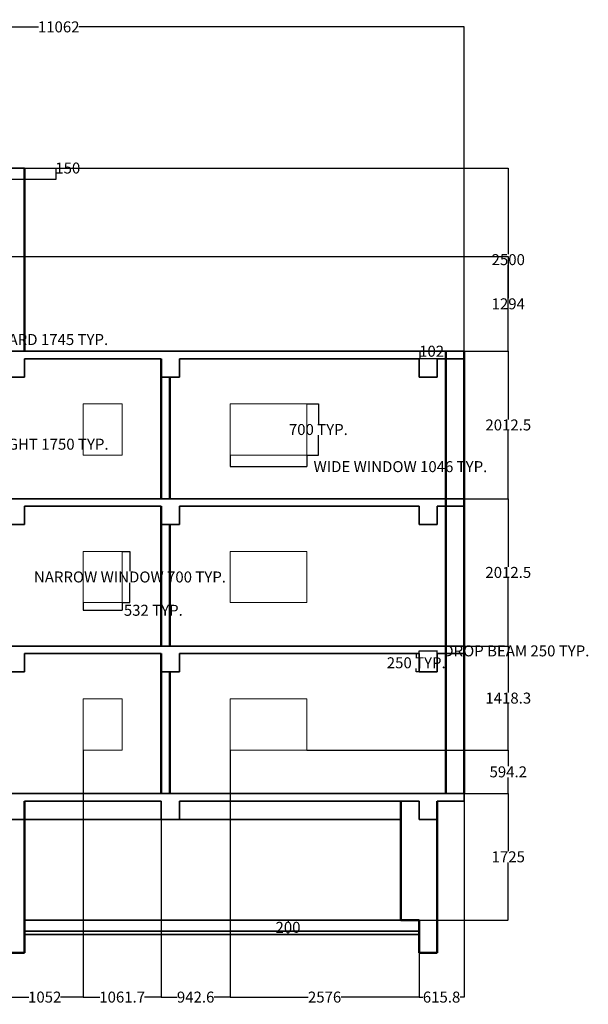
# Model space of a CAD drawing. Units: millimetres. Extents: x -1193 to 12449, y -949 to 12489.
# Tile 2 of 2: x 4692 to 12449, y -949 to 12489. Entities that reach past the tile are written whole.
import ezdxf

# ---------------------------------------------------------------- set-up
doc = ezdxf.new("R2010")
doc.units = ezdxf.units.MM
doc.header["$LTSCALE"] = 12
doc.header["$MEASUREMENT"] = 0
for name, color, linetype, lineweight in [('A-ANNO-DIMS', 2, 'Continuous', 18), ('A-FLOR', 7, 'Continuous', 35), ('A-GLAZ', 4, 'Continuous', 18), ('A-ROOF', 7, 'Continuous', 35), ('A-WALL', 7, 'Continuous', 50), ('S-BEAM', 1, 'Continuous', 35), ('S-COLS', 1, 'Continuous', 50), ('S-FNDN', 1, 'Continuous', 50)]:
    doc.layers.add(name, color=color, linetype=linetype, lineweight=lineweight)
doc.styles.get("Standard").update_dxf_attribs({"font": 'arial.ttf'})
doc.dimstyles.get("Standard").update_dxf_attribs({"dimtxt": 150, "dimasz": 0.18, "dimexe": 0.18, "dimexo": 0.0625, "dimgap": 0.09, "dimtad": 0, "dimtih": 1, "dimtoh": 1, "dimdec": 0, "dimzin": 0, "dimdsep": 46, "dimtxsty": 'Standard', "dimcen": 0.09, "dimadec": 0, "dimazin": 0, "dimtfac": 1, "dimtdec": 0, "dimtofl": 0, "dimtmove": 0, "dimatfit": 3, "dimfxl": 1, "dimtolj": 1, "dimtzin": 0, "dimarcsym": 0})

# ---------------------------------------------------------------- blocks, each defined once
blk = doc.blocks.new('*D4')
at = {"layer": 'A-ANNO-DIMS', "color": 0, "lineweight": -2, "ltscale": 8, "transparency": 16777216}
for p, q in [((8280.605673072427, 201.7493925244232), (8352.514123086432, 201.7493925244232)), ((8352.334123086432, 201.5693925244232), (8352.334123086432, 178.4253406826769)), ((8280.605673072427, 1.749392524423062), (8352.514123086432, 1.749392524423074)), ((8352.334123086432, 1.929392524423073), (8352.334123086432, 25.07344436616934))]:
    blk.add_line(p, q, dxfattribs=at)
at = {"layer": 'A-ANNO-DIMS', "color": 0, "ltscale": 8, "transparency": 16777216}
for points in [[(8352.304123086431, 201.5693925244232), (8352.364123086432, 201.5693925244232), (8352.334123086432, 201.7493925244232)], [(8352.304123086431, 1.929392524423073), (8352.364123086432, 1.929392524423073), (8352.334123086432, 1.749392524423073)]]:
    blk.add_solid(points, dxfattribs=at)
at = {"layer": 'Defpoints', "color": 0, "ltscale": 8, "transparency": 16777216}
for p in [(8280.543173072427, 201.7493925244232), (8280.543173072427, 1.749392524423062), (8352.334123086432, 1.749392524423073)]:
    blk.add_point(p, dxfattribs=at)
at = {"layer": 'A-ANNO-DIMS', "color": 0, "ltscale": 8, "transparency": 16777216, "insert": (8352.33412308643, 101.7493925244207), "char_height": 150, "attachment_point": 5}
blk.add_mtext('\\A1;200', dxfattribs=at)
blk = doc.blocks.new('*D7')
at = {"layer": 'A-ANNO-DIMS', "color": 0, "lineweight": -2, "ltscale": 8, "transparency": 16777216}
for p, q in [((4507.073797115451, 10464.24939252442), (5189.656778496646, 10464.24939252442)), ((5189.476778496646, 10464.24939252442), (5189.476778496646, 10464.42939252443)), ((5189.476778496646, 10464.42939252443), (5189.656778496646, 10464.42939252443)), ((5189.476778496646, 10314.42939252443), (5189.476778496646, 10464.06939252442)), ((4507.073797115451, 10314.24939252443), (5189.656778496646, 10314.24939252443))]:
    blk.add_line(p, q, dxfattribs=at)
at = {"layer": 'A-ANNO-DIMS', "color": 0, "ltscale": 8, "transparency": 16777216}
for points in [[(5189.446778496646, 10464.06939252442), (5189.506778496646, 10464.06939252442), (5189.476778496646, 10464.24939252442)], [(5189.446778496646, 10314.42939252443), (5189.506778496646, 10314.42939252443), (5189.476778496646, 10314.24939252443)]]:
    blk.add_solid(points, dxfattribs=at)
at = {"layer": 'Defpoints', "color": 0, "ltscale": 8, "transparency": 16777216}
for p in [(4507.01129711545, 10464.24939252442), (5189.476778496646, 10464.24939252442), (4507.01129711545, 10314.24939252443)]:
    blk.add_point(p, dxfattribs=at)
at = {"layer": 'A-ANNO-DIMS', "color": 0, "ltscale": 8, "transparency": 16777216, "insert": (5348.136955849991, 10464.42939252442), "char_height": 150, "attachment_point": 5}
blk.add_mtext('\\A1;150', dxfattribs=at)
blk = doc.blocks.new('WIN-NARROW-ELEV')
at = {"ltscale": 8}
blk.add_lwpolyline([(0, 699.7375599981679), (532.1917753348897, 699.7375599981679), (532.1917753348897, 0), (0, 0)], close=True, dxfattribs=at)
blk = doc.blocks.new('WIN-WIDE-ELEV')
at = {"ltscale": 8}
blk.add_lwpolyline([(0, 699.7375599981679), (1046.240615612791, 699.7375599981679), (1046.240615612791, 0), (0, 0)], close=True, dxfattribs=at)
blk = doc.blocks.new('BEAM-DROP-250x250')
for p, q in [((0, 250), (0, 0)), ((250, 0), (250, 250)), ((0, 0), (250, 0))]:
    blk.add_line(p, q)
blk = doc.blocks.new('*D15')
at = {"layer": 'A-ANNO-DIMS', "color": 0, "lineweight": -2, "ltscale": 8, "transparency": 16777216}
for p, q in [((10139.29307540164, 3837.311892524423), (10139.29307540164, 3874.929392524423)), ((10139.47307540164, 3874.749392524423), (10389.11307540164, 3874.749392524423)), ((10389.29307540164, 3837.311892524423), (10389.29307540164, 3874.929392524423)), ((10389.29307540164, 3874.749392524423), (10389.47307540164, 3874.749392524423))]:
    blk.add_line(p, q, dxfattribs=at)
at = {"layer": 'A-ANNO-DIMS', "color": 0, "ltscale": 8, "transparency": 16777216}
for points in [[(10139.47307540164, 3874.779392524423), (10139.47307540164, 3874.719392524422), (10139.29307540164, 3874.749392524423)], [(10389.11307540164, 3874.779392524423), (10389.11307540164, 3874.719392524422), (10389.29307540164, 3874.749392524423)]]:
    blk.add_solid(points, dxfattribs=at)
at = {"layer": 'Defpoints', "color": 0, "ltscale": 8, "transparency": 16777216}
for p in [(10139.29307540164, 3837.249392524423), (10389.29307540164, 3874.749392524423), (10389.29307540164, 3837.249392524423)]:
    blk.add_point(p, dxfattribs=at)
at = {"layer": 'A-ANNO-DIMS', "color": 0, "ltscale": 8, "transparency": 16777216, "insert": (11467.03579027203, 3874.749392524423), "char_height": 150, "attachment_point": 5}
blk.add_mtext('\\A1;DROP BEAM 250 TYP.', dxfattribs=at)
blk = doc.blocks.new('*D16')
at = {"layer": 'A-ANNO-DIMS', "color": 0, "lineweight": -2, "ltscale": 8, "transparency": 16777216}
for p, q in [((10139.23057540164, 3837.249392524425), (10101.61307540164, 3837.249392524425)), ((10101.79307540165, 3837.069392524425), (10101.79307540165, 3788.925340682679)), ((10101.79307540165, 3587.429392524425), (10101.79307540165, 3635.573444366171)), ((10139.23057540164, 3587.249392524425), (10101.61307540164, 3587.249392524425))]:
    blk.add_line(p, q, dxfattribs=at)
at = {"layer": 'A-ANNO-DIMS', "color": 0, "ltscale": 8, "transparency": 16777216}
for points in [[(10101.76307540164, 3837.069392524425), (10101.82307540165, 3837.069392524425), (10101.79307540165, 3837.249392524425)], [(10101.76307540164, 3587.429392524425), (10101.82307540165, 3587.429392524425), (10101.79307540165, 3587.249392524425)]]:
    blk.add_solid(points, dxfattribs=at)
at = {"layer": 'Defpoints', "color": 0, "ltscale": 8, "transparency": 16777216}
for p in [(10101.79307540165, 3837.249392524425), (10139.29307540164, 3837.249392524425), (10139.29307540164, 3587.249392524425)]:
    blk.add_point(p, dxfattribs=at)
at = {"layer": 'A-ANNO-DIMS', "color": 0, "ltscale": 8, "transparency": 16777216, "insert": (10101.79307540164, 3712.249392524422), "char_height": 150, "attachment_point": 5}
blk.add_mtext('\\A1;250 TYP.', dxfattribs=at)
blk = doc.blocks.new('*D19')
at = {"layer": 'A-ANNO-DIMS', "color": 0, "lineweight": -2, "ltscale": 8, "transparency": 16777216}
for p, q in [((1557.011297115448, 6957.936892524424), (1557.011297115448, 6695.319392524424)), ((3307.01129711545, 6957.936892524424), (3307.01129711545, 6695.319392524424)), ((1557.191297115448, 6695.499392524424), (3306.831297115449, 6695.499392524424)), ((3307.01129711545, 6695.499392524424), (3307.19129711545, 6695.499392524424))]:
    blk.add_line(p, q, dxfattribs=at)
at = {"layer": 'A-ANNO-DIMS', "color": 0, "ltscale": 8, "transparency": 16777216}
for points in [[(1557.191297115448, 6695.529392524425), (1557.191297115448, 6695.469392524424), (1557.011297115448, 6695.499392524424)], [(3306.831297115449, 6695.529392524425), (3306.831297115449, 6695.469392524424), (3307.01129711545, 6695.499392524424)]]:
    blk.add_solid(points, dxfattribs=at)
at = {"layer": 'Defpoints', "color": 0, "ltscale": 8, "transparency": 16777216}
for p in [(1557.011297115448, 6957.999392524424), (3307.01129711545, 6957.999392524424), (3307.01129711545, 6695.499392524424)]:
    blk.add_point(p, dxfattribs=at)
at = {"layer": 'A-ANNO-DIMS', "color": 0, "ltscale": 8, "transparency": 16777216, "insert": (4652.318814168655, 6695.499392524424), "char_height": 150, "attachment_point": 5}
blk.add_mtext('\\A1;RETURN FLIGHT 1750 TYP.', dxfattribs=at)
blk = doc.blocks.new('*D21')
at = {"layer": 'A-ANNO-DIMS', "color": 0, "lineweight": -2, "ltscale": 8, "transparency": 16777216}
for p, q in [((1557.011297115448, 7862.311892524418), (1557.011297115448, 8124.17479182941)), ((1557.191297115448, 8123.99479182941), (3301.800625815397, 8123.99479182941)), ((3301.980625815397, 7862.311892524418), (3301.980625815397, 8124.17479182941)), ((3301.980625815397, 8123.99479182941), (3302.160625815397, 8123.99479182941))]:
    blk.add_line(p, q, dxfattribs=at)
at = {"layer": 'A-ANNO-DIMS', "color": 0, "ltscale": 8, "transparency": 16777216}
for points in [[(1557.191297115448, 8124.024791829411), (1557.191297115448, 8123.964791829411), (1557.011297115448, 8123.99479182941)], [(3301.800625815397, 8124.024791829411), (3301.800625815397, 8123.964791829411), (3301.980625815397, 8123.99479182941)]]:
    blk.add_solid(points, dxfattribs=at)
at = {"layer": 'Defpoints', "color": 0, "ltscale": 8, "transparency": 16777216}
for p in [(3301.980625815397, 8123.99479182941), (1557.011297115448, 7862.249392524418), (3301.980625815397, 7862.249392524418)]:
    blk.add_point(p, dxfattribs=at)
at = {"layer": 'A-ANNO-DIMS', "color": 0, "ltscale": 8, "transparency": 16777216, "insert": (4653.120339321535, 8123.99479182941), "char_height": 150, "attachment_point": 5}
blk.add_mtext('\\A1;RETURN GUARD 1745 TYP.', dxfattribs=at)
blk = doc.blocks.new('*D23')
at = {"layer": 'A-ANNO-DIMS', "color": 0, "lineweight": -2, "ltscale": 8, "transparency": 16777216}
for p, q in [((6091.350578652216, 5233.211343509282), (6196.428712651947, 5233.211343509282)), ((6196.248712651946, 5233.031343509281), (6196.248712651946, 4961.041704028616)), ((6196.248712651946, 4533.653783511115), (6196.248712651946, 4805.643422991781)), ((6091.350578652216, 4533.473783511113), (6196.428712651947, 4533.473783511115))]:
    blk.add_line(p, q, dxfattribs=at)
at = {"layer": 'A-ANNO-DIMS', "color": 0, "ltscale": 8, "transparency": 16777216}
for points in [[(6196.218712651947, 5233.031343509281), (6196.278712651946, 5233.031343509281), (6196.248712651946, 5233.211343509282)], [(6196.218712651947, 4533.653783511115), (6196.278712651946, 4533.653783511115), (6196.248712651946, 4533.473783511115)]]:
    blk.add_solid(points, dxfattribs=at)
at = {"layer": 'Defpoints', "color": 0, "ltscale": 8, "transparency": 16777216}
for p in [(6091.288078652215, 5233.211343509282), (6196.248712651946, 5233.211343509282), (6091.288078652215, 4533.473783511113)]:
    blk.add_point(p, dxfattribs=at)
at = {"layer": 'A-ANNO-DIMS', "color": 0, "ltscale": 8, "transparency": 16777216, "insert": (6196.248712651946, 4883.342563510196), "char_height": 150, "attachment_point": 5}
blk.add_mtext('\\A1;NARROW WINDOW 700 TYP.', dxfattribs=at)
blk = doc.blocks.new('*D24')
at = {"layer": 'A-ANNO-DIMS', "color": 0, "lineweight": -2, "ltscale": 8, "transparency": 16777216}
for p, q in [((5559.096303317324, 4533.411283511112), (5559.096303317324, 4428.333149511386)), ((6091.288078652214, 4533.411283511112), (6091.288078652214, 4428.333149511386)), ((5559.276303317324, 4428.513149511386), (6091.108078652213, 4428.513149511386)), ((6091.288078652214, 4428.513149511386), (6091.468078652214, 4428.513149511386))]:
    blk.add_line(p, q, dxfattribs=at)
at = {"layer": 'A-ANNO-DIMS', "color": 0, "ltscale": 8, "transparency": 16777216}
for points in [[(5559.276303317324, 4428.543149511386), (5559.276303317324, 4428.483149511387), (5559.096303317324, 4428.513149511386)], [(6091.108078652213, 4428.543149511386), (6091.108078652213, 4428.483149511387), (6091.288078652214, 4428.513149511386)]]:
    blk.add_solid(points, dxfattribs=at)
at = {"layer": 'Defpoints', "color": 0, "ltscale": 8, "transparency": 16777216}
for p in [(5559.096303317324, 4533.473783511111), (6091.288078652214, 4533.473783511111), (6091.288078652214, 4428.513149511386)]:
    blk.add_point(p, dxfattribs=at)
at = {"layer": 'A-ANNO-DIMS', "color": 0, "ltscale": 8, "transparency": 16777216, "insert": (6514.903917669949, 4428.513149511386), "char_height": 150, "attachment_point": 5}
blk.add_mtext('\\A1;532 TYP.', dxfattribs=at)
blk = doc.blocks.new('*D25')
at = {"layer": 'A-ANNO-DIMS', "color": 0, "lineweight": -2, "ltscale": 8, "transparency": 16777216}
for p, q in [((7563.33082917866, 6545.911283511111), (7563.33082917866, 6388.857691169192)), ((8609.57144479145, 6545.911283511111), (8609.57144479145, 6388.857691169192)), ((7563.51082917866, 6389.037691169193), (8609.39144479145, 6389.037691169193)), ((8609.57144479145, 6389.037691169193), (8609.75144479145, 6389.037691169193))]:
    blk.add_line(p, q, dxfattribs=at)
at = {"layer": 'A-ANNO-DIMS', "color": 0, "ltscale": 8, "transparency": 16777216}
for points in [[(7563.51082917866, 6389.067691169192), (7563.51082917866, 6389.007691169194), (7563.33082917866, 6389.037691169193)], [(8609.39144479145, 6389.067691169192), (8609.39144479145, 6389.007691169194), (8609.57144479145, 6389.037691169193)]]:
    blk.add_solid(points, dxfattribs=at)
at = {"layer": 'Defpoints', "color": 0, "ltscale": 8, "transparency": 16777216}
for p in [(7563.33082917866, 6545.973783511112), (8609.57144479145, 6545.973783511112), (8609.57144479145, 6389.037691169193)]:
    blk.add_point(p, dxfattribs=at)
at = {"layer": 'A-ANNO-DIMS', "color": 0, "ltscale": 8, "transparency": 16777216, "insert": (9886.018116005638, 6389.037691169193), "char_height": 150, "attachment_point": 5}
blk.add_mtext('\\A1;WIDE WINDOW 1046 TYP.', dxfattribs=at)
blk = doc.blocks.new('*D26')
at = {"layer": 'A-ANNO-DIMS', "color": 0, "lineweight": -2, "ltscale": 8, "transparency": 16777216}
for p, q in [((8609.633944791454, 7245.711343509284), (8766.687537133377, 7245.711343509284)), ((8766.507537133377, 7245.531343509283), (8766.507537133377, 6972.518511668453)), ((8766.507537133377, 6546.153783511115), (8766.507537133377, 6819.166615351945)), ((8609.633944791454, 6545.973783511115), (8766.687537133377, 6545.973783511115))]:
    blk.add_line(p, q, dxfattribs=at)
at = {"layer": 'A-ANNO-DIMS', "color": 0, "ltscale": 8, "transparency": 16777216}
for points in [[(8766.477537133376, 7245.531343509283), (8766.53753713338, 7245.531343509283), (8766.507537133377, 7245.711343509284)], [(8766.477537133376, 6546.153783511115), (8766.53753713338, 6546.153783511115), (8766.507537133377, 6545.973783511115)]]:
    blk.add_solid(points, dxfattribs=at)
at = {"layer": 'Defpoints', "color": 0, "ltscale": 8, "transparency": 16777216}
for p in [(8609.571444791454, 7245.711343509284), (8766.507537133377, 7245.711343509284), (8609.571444791454, 6545.973783511115)]:
    blk.add_point(p, dxfattribs=at)
at = {"layer": 'A-ANNO-DIMS', "color": 0, "ltscale": 8, "transparency": 16777216, "insert": (8766.507537133377, 6895.842563510194), "char_height": 150, "attachment_point": 5}
blk.add_mtext('\\A1;700 TYP.', dxfattribs=at)
blk = doc.blocks.new('*D27')
at = {"layer": 'A-ANNO-DIMS', "color": 0, "lineweight": -2, "ltscale": 8, "transparency": 16777216}
for p, q in [((-307.014113, 8654.059893999998), (-307.0141129999998, 12390.66548)), ((-306.8341129999998, 12390.48548), (4949.545781004093, 12390.48548)), ((10754.946057, 12390.48548), (5498.566162995907, 12390.48548)), ((10755.126057, 7964.311893), (10755.126057, 12390.66548))]:
    blk.add_line(p, q, dxfattribs=at)
at = {"layer": 'A-ANNO-DIMS', "color": 0, "ltscale": 8, "transparency": 16777216}
for points in [[(-306.8341129999998, 12390.51548), (-306.8341129999998, 12390.45548), (-307.0141129999998, 12390.48548)], [(10754.946057, 12390.51548), (10754.946057, 12390.45548), (10755.126057, 12390.48548)]]:
    blk.add_solid(points, dxfattribs=at)
at = {"layer": 'Defpoints', "color": 0, "ltscale": 8, "transparency": 16777216}
for p in [(10755.126057, 12390.48548), (-307.014113, 8653.997393999998), (10755.126057, 7964.249393)]:
    blk.add_point(p, dxfattribs=at)
at = {"layer": 'A-ANNO-DIMS', "color": 0, "ltscale": 8, "transparency": 16777216, "insert": (5224.055972, 12390.48548), "char_height": 150, "attachment_point": 5}
blk.add_mtext('\\A1;11062', dxfattribs=at)
blk = doc.blocks.new('*D30')
at = {"layer": 'A-ANNO-DIMS', "color": 0, "lineweight": -2, "ltscale": 8, "transparency": 16777216}
for p, q in [((5559.096303, 2520.911284), (5559.096303, -850.4306069999998)), ((4507.011297, -248.313107), (4507.011297, -850.430607)), ((4507.191297000001, -850.250607), (4816.814413915416, -850.250607)), ((5558.916303, -850.250607), (5249.293186084583, -850.250607))]:
    blk.add_line(p, q, dxfattribs=at)
at = {"layer": 'A-ANNO-DIMS', "color": 0, "ltscale": 8, "transparency": 16777216}
for points in [[(4507.191297000001, -850.2206069999999), (4507.191297000001, -850.280607), (4507.011297, -850.250607)], [(5558.916303, -850.2206069999999), (5558.916303, -850.280607), (5559.096303, -850.250607)]]:
    blk.add_solid(points, dxfattribs=at)
at = {"layer": 'Defpoints', "color": 0, "ltscale": 8, "transparency": 16777216}
for p in [(5559.096303, 2520.973784), (4507.011297, -248.250607), (5559.096303, -850.250607)]:
    blk.add_point(p, dxfattribs=at)
at = {"layer": 'A-ANNO-DIMS', "color": 0, "ltscale": 8, "transparency": 16777216, "insert": (5033.0538, -850.250607), "char_height": 150, "attachment_point": 5}
blk.add_mtext('\\A1;1052', dxfattribs=at)
blk = doc.blocks.new('*D31')
at = {"layer": 'A-ANNO-DIMS', "color": 0, "lineweight": -2, "ltscale": 8, "transparency": 16777216}
for p, q in [((5559.096303, 2520.911284), (5559.096303, -850.4306069999998)), ((6620.771954, 1575.086893), (6620.771954, -850.4306069999994)), ((5559.276303, -850.250607), (5785.546720587313, -850.250607)), ((6620.591954, -850.250607), (6394.321536412687, -850.250607))]:
    blk.add_line(p, q, dxfattribs=at)
at = {"layer": 'A-ANNO-DIMS', "color": 0, "ltscale": 8, "transparency": 16777216}
for points in [[(5559.276303, -850.2206069999999), (5559.276303, -850.280607), (5559.096303, -850.250607)], [(6620.591954, -850.2206069999999), (6620.591954, -850.280607), (6620.771954, -850.250607)]]:
    blk.add_solid(points, dxfattribs=at)
at = {"layer": 'Defpoints', "color": 0, "ltscale": 8, "transparency": 16777216}
for p in [(5559.096303, 2520.973784), (6620.771954, 1575.149393), (6620.771954, -850.250607)]:
    blk.add_point(p, dxfattribs=at)
at = {"layer": 'A-ANNO-DIMS', "color": 0, "ltscale": 8, "transparency": 16777216, "insert": (6089.9341285, -850.250607), "char_height": 150, "attachment_point": 5}
blk.add_mtext('\\A1;1061.7', dxfattribs=at)
blk = doc.blocks.new('*D32')
at = {"layer": 'A-ANNO-DIMS', "color": 0, "lineweight": -2, "ltscale": 8, "transparency": 16777216}
for p, q in [((7563.330829, 2520.911284), (7563.330829, -850.4306069999998)), ((6620.771954, 1575.086893), (6620.771954, -850.4306069999994)), ((6620.951954, -850.250607), (6838.925920831513, -850.250607)), ((7563.150829, -850.250607), (7345.176862168486, -850.250607))]:
    blk.add_line(p, q, dxfattribs=at)
at = {"layer": 'A-ANNO-DIMS', "color": 0, "ltscale": 8, "transparency": 16777216}
for points in [[(6620.951954, -850.2206069999999), (6620.951954, -850.280607), (6620.771954, -850.250607)], [(7563.150829, -850.2206069999999), (7563.150829, -850.280607), (7563.330829, -850.250607)]]:
    blk.add_solid(points, dxfattribs=at)
at = {"layer": 'Defpoints', "color": 0, "ltscale": 8, "transparency": 16777216}
for p in [(7563.330829, 2520.973784), (6620.771954, 1575.149393), (7563.330829, -850.250607)]:
    blk.add_point(p, dxfattribs=at)
at = {"layer": 'A-ANNO-DIMS', "color": 0, "ltscale": 8, "transparency": 16777216, "insert": (7092.0513915, -850.250607), "char_height": 150, "attachment_point": 5}
blk.add_mtext('\\A1;942.6', dxfattribs=at)
blk = doc.blocks.new('*D33')
at = {"layer": 'A-ANNO-DIMS', "color": 0, "lineweight": -2, "ltscale": 8, "transparency": 16777216}
for p, q in [((7563.330829, 2520.911284), (7563.330829, -850.4306069999998)), ((10139.293075, -248.313107), (10139.293075, -850.430607)), ((7563.510829000001, -850.250607), (8626.017313527967, -850.250607)), ((10139.113075, -850.250607), (9076.606590472033, -850.250607))]:
    blk.add_line(p, q, dxfattribs=at)
at = {"layer": 'A-ANNO-DIMS', "color": 0, "ltscale": 8, "transparency": 16777216}
for points in [[(7563.510829000001, -850.2206069999999), (7563.510829000001, -850.280607), (7563.330829, -850.250607)], [(10139.113075, -850.2206069999999), (10139.113075, -850.280607), (10139.293075, -850.250607)]]:
    blk.add_solid(points, dxfattribs=at)
at = {"layer": 'Defpoints', "color": 0, "ltscale": 8, "transparency": 16777216}
for p in [(7563.330829, 2520.973784), (10139.293075, -248.250607), (10139.293075, -850.250607)]:
    blk.add_point(p, dxfattribs=at)
at = {"layer": 'A-ANNO-DIMS', "color": 0, "ltscale": 8, "transparency": 16777216, "insert": (8851.311952000002, -850.250607), "char_height": 150, "attachment_point": 5}
blk.add_mtext('\\A1;2576', dxfattribs=at)
blk = doc.blocks.new('*D34')
at = {"layer": 'A-ANNO-DIMS', "color": 0, "lineweight": -2, "ltscale": 8, "transparency": 16777216}
for p, q in [((10755.126057, 1825.086893), (10755.126057, -850.4306069999994)), ((10139.293075, -248.313107), (10139.293075, -850.430607)), ((10139.473075, -850.250607), (10193.47017991541, -850.250607)), ((10754.946057, -850.250607), (10700.94895208458, -850.250607))]:
    blk.add_line(p, q, dxfattribs=at)
at = {"layer": 'A-ANNO-DIMS', "color": 0, "ltscale": 8, "transparency": 16777216}
for points in [[(10139.473075, -850.2206069999999), (10139.473075, -850.280607), (10139.293075, -850.250607)], [(10754.946057, -850.2206069999999), (10754.946057, -850.280607), (10755.126057, -850.250607)]]:
    blk.add_solid(points, dxfattribs=at)
at = {"layer": 'Defpoints', "color": 0, "ltscale": 8, "transparency": 16777216}
for p in [(10755.126057, 1825.149393), (10139.293075, -248.250607), (10755.126057, -850.250607)]:
    blk.add_point(p, dxfattribs=at)
at = {"layer": 'A-ANNO-DIMS', "color": 0, "ltscale": 8, "transparency": 16777216, "insert": (10447.209566, -850.250607), "char_height": 150, "attachment_point": 5}
blk.add_mtext('\\A1;615.8', dxfattribs=at)
blk = doc.blocks.new('*D35')
at = {"layer": 'A-ANNO-DIMS', "color": 0, "lineweight": -2, "ltscale": 8, "transparency": 16777216}
for p, q in [((10755.188557, 1926.749393000001), (11357.306057, 1926.749393000001)), ((11357.126057, 1926.569393000001), (11357.126057, 1140.925341158254)), ((11357.126057, 201.9293930000003), (11357.126057, 987.5734448417468)), ((10139.355575, 201.7493930000001), (11357.306057, 201.7493930000003))]:
    blk.add_line(p, q, dxfattribs=at)
at = {"layer": 'A-ANNO-DIMS', "color": 0, "ltscale": 8, "transparency": 16777216}
for points in [[(11357.096057, 1926.569393000001), (11357.15605700001, 1926.569393000001), (11357.126057, 1926.749393000001)], [(11357.096057, 201.9293930000003), (11357.15605700001, 201.9293930000003), (11357.126057, 201.7493930000003)]]:
    blk.add_solid(points, dxfattribs=at)
at = {"layer": 'Defpoints', "color": 0, "ltscale": 8, "transparency": 16777216}
for p in [(10755.126057, 1926.749393000001), (11357.126057, 1926.749393000001), (10139.293075, 201.7493930000001)]:
    blk.add_point(p, dxfattribs=at)
at = {"layer": 'A-ANNO-DIMS', "color": 0, "ltscale": 8, "transparency": 16777216, "insert": (11357.126057, 1064.249392999997), "char_height": 150, "attachment_point": 5}
blk.add_mtext('\\A1;1725', dxfattribs=at)
blk = doc.blocks.new('*D36')
at = {"layer": 'A-ANNO-DIMS', "color": 0, "lineweight": -2, "ltscale": 8, "transparency": 16777216}
for p, q in [((8609.633945000003, 2520.973784000001), (11357.306057, 2520.973784000002)), ((11357.126057, 2520.793784000002), (11357.126057, 2300.537536658255)), ((11357.126057, 1926.929393000001), (11357.126057, 2147.185640341747)), ((10755.188557, 1926.749393000001), (11357.306057, 1926.749393000001))]:
    blk.add_line(p, q, dxfattribs=at)
at = {"layer": 'A-ANNO-DIMS', "color": 0, "ltscale": 8, "transparency": 16777216}
for points in [[(11357.096057, 2520.793784000002), (11357.15605700001, 2520.793784000002), (11357.126057, 2520.973784000002)], [(11357.096057, 1926.929393000001), (11357.15605700001, 1926.929393000001), (11357.126057, 1926.749393000001)]]:
    blk.add_solid(points, dxfattribs=at)
at = {"layer": 'Defpoints', "color": 0, "ltscale": 8, "transparency": 16777216}
for p in [(8609.571445000003, 2520.973784000001), (11357.126057, 2520.973784000002), (10755.126057, 1926.749393000001)]:
    blk.add_point(p, dxfattribs=at)
at = {"layer": 'A-ANNO-DIMS', "color": 0, "ltscale": 8, "transparency": 16777216, "insert": (11357.126057, 2223.861588499997), "char_height": 150, "attachment_point": 5}
blk.add_mtext('\\A1;594.2', dxfattribs=at)
blk = doc.blocks.new('*D37')
at = {"layer": 'A-ANNO-DIMS', "color": 0, "lineweight": -2, "ltscale": 8, "transparency": 16777216}
for p, q in [((10755.188557, 3939.249393000002), (11357.306057, 3939.249393000002)), ((11357.126057, 3939.069393000003), (11357.126057, 3306.838696276265)), ((11357.126057, 2521.153784000002), (11357.126057, 3153.38448072374)), ((8609.633945000003, 2520.973784000001), (11357.306057, 2520.973784000002))]:
    blk.add_line(p, q, dxfattribs=at)
at = {"layer": 'A-ANNO-DIMS', "color": 0, "ltscale": 8, "transparency": 16777216}
for points in [[(11357.096057, 3939.069393000003), (11357.15605700001, 3939.069393000003), (11357.126057, 3939.249393000002)], [(11357.096057, 2521.153784000002), (11357.15605700001, 2521.153784000002), (11357.126057, 2520.973784000002)]]:
    blk.add_solid(points, dxfattribs=at)
at = {"layer": 'Defpoints', "color": 0, "ltscale": 8, "transparency": 16777216}
for p in [(10755.126057, 3939.249393000002), (11357.126057, 3939.249393000002), (8609.571445000003, 2520.973784000001)]:
    blk.add_point(p, dxfattribs=at)
at = {"layer": 'A-ANNO-DIMS', "color": 0, "ltscale": 8, "transparency": 16777216, "insert": (11357.126057, 3230.111588499998), "char_height": 150, "attachment_point": 5}
blk.add_mtext('\\A1;1418.3', dxfattribs=at)
blk = doc.blocks.new('*D38')
at = {"layer": 'A-ANNO-DIMS', "color": 0, "lineweight": -2, "ltscale": 8, "transparency": 16777216}
for p, q in [((10755.188557, 5951.749393000002), (11357.306057, 5951.749393000002)), ((11357.126057, 5951.569393000002), (11357.126057, 5022.175341158256)), ((11357.12605700001, 3939.429393000003), (11357.126057, 4868.823444841748)), ((10755.188557, 3939.249393000002), (11357.30605700001, 3939.249393000002))]:
    blk.add_line(p, q, dxfattribs=at)
at = {"layer": 'A-ANNO-DIMS', "color": 0, "ltscale": 8, "transparency": 16777216}
for points in [[(11357.096057, 5951.569393000002), (11357.15605700001, 5951.569393000002), (11357.126057, 5951.749393000002)], [(11357.09605700001, 3939.429393000003), (11357.15605700001, 3939.429393000003), (11357.12605700001, 3939.249393000002)]]:
    blk.add_solid(points, dxfattribs=at)
at = {"layer": 'Defpoints', "color": 0, "ltscale": 8, "transparency": 16777216}
for p in [(10755.126057, 5951.749393000002), (11357.126057, 5951.749393000002), (10755.126057, 3939.249393000002)]:
    blk.add_point(p, dxfattribs=at)
at = {"layer": 'A-ANNO-DIMS', "color": 0, "ltscale": 8, "transparency": 16777216, "insert": (11357.126057, 4945.499392999997), "char_height": 150, "attachment_point": 5}
blk.add_mtext('\\A1;2012.5', dxfattribs=at)
blk = doc.blocks.new('*D39')
at = {"layer": 'A-ANNO-DIMS', "color": 0, "lineweight": -2, "ltscale": 8, "transparency": 16777216}
for p, q in [((10755.188557, 7964.249393000004), (11357.306057, 7964.249393000004)), ((11357.126057, 7964.069393000004), (11357.126057, 7034.675341158257)), ((11357.126057, 5951.929393000003), (11357.126057, 6881.323444841749)), ((10755.188557, 5951.749393000002), (11357.306057, 5951.749393000002))]:
    blk.add_line(p, q, dxfattribs=at)
at = {"layer": 'A-ANNO-DIMS', "color": 0, "ltscale": 8, "transparency": 16777216}
for points in [[(11357.096057, 7964.069393000004), (11357.15605700001, 7964.069393000004), (11357.126057, 7964.249393000004)], [(11357.096057, 5951.929393000003), (11357.15605700001, 5951.929393000003), (11357.126057, 5951.749393000002)]]:
    blk.add_solid(points, dxfattribs=at)
at = {"layer": 'Defpoints', "color": 0, "ltscale": 8, "transparency": 16777216}
for p in [(10755.126057, 7964.249393000004), (11357.126057, 7964.249393000004), (10755.126057, 5951.749393000002)]:
    blk.add_point(p, dxfattribs=at)
at = {"layer": 'A-ANNO-DIMS', "color": 0, "ltscale": 8, "transparency": 16777216, "insert": (11357.126057, 6957.999392999997), "char_height": 150, "attachment_point": 5}
blk.add_mtext('\\A1;2012.5', dxfattribs=at)
blk = doc.blocks.new('*D40')
at = {"layer": 'A-ANNO-DIMS', "color": 0, "lineweight": -2, "ltscale": 8, "transparency": 16777216}
for p, q in [((4757.073797000002, 10464.249393), (11357.306057, 10464.249393)), ((11357.126057, 10464.069393), (11357.126057, 9290.925341158258)), ((11357.126057, 7964.429393000006), (11357.126057, 9137.57344484175)), ((4757.073797000002, 7964.249393000004), (11357.306057, 7964.249393000006))]:
    blk.add_line(p, q, dxfattribs=at)
at = {"layer": 'A-ANNO-DIMS', "color": 0, "ltscale": 8, "transparency": 16777216}
for points in [[(11357.096057, 10464.069393), (11357.15605700001, 10464.069393), (11357.126057, 10464.249393)], [(11357.096057, 7964.429393000006), (11357.15605700001, 7964.429393000006), (11357.126057, 7964.249393000006)]]:
    blk.add_solid(points, dxfattribs=at)
at = {"layer": 'Defpoints', "color": 0, "ltscale": 8, "transparency": 16777216}
for p in [(4757.011297000001, 10464.249393), (11357.126057, 10464.249393), (4757.011297000001, 7964.249393000004)]:
    blk.add_point(p, dxfattribs=at)
at = {"layer": 'A-ANNO-DIMS', "color": 0, "ltscale": 8, "transparency": 16777216, "insert": (11357.126057, 9214.249393000002), "char_height": 150, "attachment_point": 5}
blk.add_mtext('\\A1;2500', dxfattribs=at)
blk = doc.blocks.new('*D44')
at = {"layer": 'A-ANNO-DIMS', "color": 0, "lineweight": -2, "ltscale": 8, "transparency": 16777216}
for p, q in [((4507.073797000002, 9258.211344000001), (11357.306057, 9258.211344000001)), ((11357.126057, 9258.031344000003), (11357.126057, 8687.906316658258)), ((11357.126057, 7964.429393000006), (11357.126057, 8534.55442034175)), ((4507.073797000002, 7964.249393000004), (11357.306057, 7964.249393000006))]:
    blk.add_line(p, q, dxfattribs=at)
at = {"layer": 'A-ANNO-DIMS', "color": 0, "ltscale": 8, "transparency": 16777216}
for points in [[(11357.096057, 9258.031344000003), (11357.15605700001, 9258.031344000003), (11357.126057, 9258.211344000001)], [(11357.096057, 7964.429393000006), (11357.15605700001, 7964.429393000006), (11357.126057, 7964.249393000006)]]:
    blk.add_solid(points, dxfattribs=at)
at = {"layer": 'Defpoints', "color": 0, "ltscale": 8, "transparency": 16777216}
for p in [(4507.011297000001, 9258.211344000001), (11357.126057, 9258.211344000001), (4507.011297000001, 7964.249393000004)]:
    blk.add_point(p, dxfattribs=at)
at = {"layer": 'A-ANNO-DIMS', "color": 0, "ltscale": 8, "transparency": 16777216, "insert": (11357.126057, 8611.2303685), "char_height": 150, "attachment_point": 5}
blk.add_mtext('\\A1;1294', dxfattribs=at)
blk = doc.blocks.new('*D50')
at = {"layer": 'A-ANNO-DIMS', "color": 0, "lineweight": -2, "ltscale": 8, "transparency": 16777216}
for p, q in [((10755.063557, 7964.249393000004), (10152.946057, 7964.249393000002)), ((10153.12605700001, 7964.249393000002), (10153.12605700001, 7964.429393000003)), ((10153.12605700001, 7964.429393000003), (10153.306057, 7964.429393000003)), ((10153.12605700001, 7862.429393000003), (10153.12605700001, 7964.069393000002)), ((10755.063557, 7862.249393000003), (10152.946057, 7862.249393000003))]:
    blk.add_line(p, q, dxfattribs=at)
at = {"layer": 'A-ANNO-DIMS', "color": 0, "ltscale": 8, "transparency": 16777216}
for points in [[(10153.096057, 7964.069393000002), (10153.15605700001, 7964.069393000002), (10153.12605700001, 7964.249393000002)], [(10153.096057, 7862.429393000003), (10153.15605700001, 7862.429393000003), (10153.12605700001, 7862.249393000003)]]:
    blk.add_solid(points, dxfattribs=at)
at = {"layer": 'Defpoints', "color": 0, "ltscale": 8, "transparency": 16777216}
for p in [(10153.12605700001, 7964.249393000002), (10755.126057, 7964.249393000004), (10755.126057, 7862.249393000003)]:
    blk.add_point(p, dxfattribs=at)
at = {"layer": 'A-ANNO-DIMS', "color": 0, "ltscale": 8, "transparency": 16777216, "insert": (10311.27463817326, 7964.429392999999), "char_height": 150, "attachment_point": 5}
blk.add_mtext('\\A1;102', dxfattribs=at)

msp = doc.modelspace()

# ---------------------------------------------------------------- linework, layer by layer
at = {"layer": 'A-FLOR', "ltscale": 8}
for p, q in [((3057.011297115449, 5951.749392524424), (10755.12605663696, 5951.749392524424)), ((4757.011297115449, 5849.749392524423), (6620.771953913441, 5849.749392524423)), ((6870.77195391344, 5849.749392524423), (10139.29307540164, 5849.749392524423)), ((10389.29307540164, 5849.749392524423), (10755.12605663696, 5849.749392524423)), ((3057.011297115449, 3939.249392524423), (10755.12605663696, 3939.249392524423)), ((4757.011297115449, 3837.249392524423), (6620.771953913441, 3837.249392524423)), ((6870.77195391344, 3837.249392524423), (10139.29307540164, 3837.249392524423)), ((10389.29307540164, 3837.249392524423), (10755.12605663696, 3837.249392524423)), ((10755.12605663696, 1825.149392524423), (10755.12605663696, 1926.749392524422)), ((10389.29307540164, 1825.149392524423), (10755.12605663696, 1825.149392524423))]:
    msp.add_line(p, q, dxfattribs=at)
at = {"layer": 'A-FLOR'}
for p, q in [((4507.011297115449, 1926.749392524423), (10755.12605663696, 1926.749392524423)), ((4757.011297115449, 1825.149392524423), (6620.771953913441, 1825.149392524423)), ((6870.771953913443, 1825.149392524423), (10139.29307540164, 1825.149392524423)), ((4757.011297115449, 201.749392524423), (10139.29307540164, 201.749392524423)), ((4757.011297115449, 51.74939252442306), (10139.29307540164, 51.74939252442306)), ((4757.011297115449, 1.749392524423061), (10139.29307540164, 1.749392524423061))]:
    msp.add_line(p, q, dxfattribs=at)
at = {"layer": 'A-ROOF', "ltscale": 8}
for p, q in [((4757.011297115449, 10464.24939252442), (107.0112971154485, 10464.24939252442)), ((3057.011297115449, 7964.249392524424), (10755.12605663696, 7964.249392524424)), ((4757.011297115449, 7862.249392524424), (6620.771953913441, 7862.249392524424)), ((6870.77195391344, 7862.249392524424), (10139.29307540164, 7862.249392524424)), ((10389.29307540164, 7862.249392524424), (10755.12605663696, 7862.249392524424))]:
    msp.add_line(p, q, dxfattribs=at)
at = {"layer": 'A-WALL', "ltscale": 8}
for p, q in [((4757.011297115449, 7964.249392524424), (4757.011297115449, 10464.24939252442)), ((10505.12605663697, 5951.749392524424), (10505.12605663697, 7964.249392524424)), ((10755.12605663696, 5951.749392524424), (10755.12605663696, 7964.249392524424)), ((6620.771953913441, 5951.749392524424), (6620.771953913441, 7862.249392524424)), ((6740.771953913442, 5951.749392524424), (6740.771953913442, 7612.249392524424)), ((10505.12605663697, 3939.249392524424), (10505.12605663697, 5951.749392524424)), ((10755.12605663696, 3939.249392524424), (10755.12605663696, 5951.749392524424)), ((6620.771953913441, 3939.249392524424), (6620.771953913441, 5849.749392524423)), ((6740.771953913442, 3939.249392524424), (6740.771953913442, 5599.749392524423)), ((10505.12605663697, 1926.749392524423), (10505.12605663697, 3939.249392524424)), ((10755.12605663696, 1926.749392524423), (10755.12605663696, 3939.249392524423)), ((6620.771953913441, 1926.749392524423), (6620.771953913441, 3837.249392524423)), ((6740.771953913442, 1926.749392524423), (6740.771953913442, 3587.249392524423))]:
    msp.add_line(p, q, dxfattribs=at)
at = {"layer": 'S-BEAM'}
msp.add_line((9889.293075401642, 1575.149392524423), (4757.011297115449, 1575.149392524423), dxfattribs=at)
at = {"layer": 'S-COLS'}
for p, q in [((4757.011297115449, 201.749392524423), (4757.011297115449, 1825.149392524423)), ((9889.293075401642, 201.749392524423), (9889.293075401642, 1825.149392524423)), ((10389.29307540164, 1825.149392524423), (10389.29307540164, 201.749392524423))]:
    msp.add_line(p, q, dxfattribs=at)
at = {"layer": 'S-FNDN'}
for p, q in [((4757.011297115449, 201.749392524423), (4757.011297115449, 1.749392524423061)), ((10139.29307540164, 201.749392524423), (9889.293075401642, 201.749392524423)), ((10139.29307540164, -248.2506074755769), (10139.29307540164, 201.749392524423)), ((10389.29307540164, 201.749392524423), (10389.29307540164, 1.749392524423061)), ((4757.011297115449, 1.749392524423061), (4757.011297115449, -248.2506074755769)), ((10389.29307540164, 1.749392524423061), (10389.29307540164, -248.2506074755769)), ((4757.011297115449, -248.2506074755769), (4507.011297115449, -248.2506074755769)), ((10389.29307540164, -248.2506074755769), (10139.29307540164, -248.2506074755769))]:
    msp.add_line(p, q, dxfattribs=at)

# ---------------------------------------------------------------- block references
at = {"layer": 'A-GLAZ'}
for name, p in [('WIN-NARROW-ELEV', (5559.096303317325, 6545.973783511112)), ('WIN-WIDE-ELEV', (7563.33082917866, 6545.973783511112)), ('WIN-NARROW-ELEV', (5559.096303317324, 4533.473783511112)), ('WIN-WIDE-ELEV', (7563.330829178659, 4533.473783511112)), ('WIN-NARROW-ELEV', (5559.096303317325, 2520.973783511112)), ('WIN-WIDE-ELEV', (7563.33082917866, 2520.973783511112))]:
    msp.add_blockref(name, p, dxfattribs=at)
at = {"layer": 'S-BEAM'}
for p in [(4507.011297115449, 7612.249392524424), (6620.771953913441, 7612.249392524424), (10139.29307540164, 7612.249392524424), (4507.011297115449, 5599.749392524423), (6620.771953913441, 5599.749392524421), (10139.29307540164, 5599.749392524421), (4507.011297115449, 3587.249392524423), (6620.771953913441, 3587.249392524423), (10139.29307540164, 3587.249392524423), (4507.011297115449, 1575.149392524423), (6620.771953913441, 1575.149392524423), (10139.29307540164, 1575.149392524423)]:
    msp.add_blockref('BEAM-DROP-250x250', p, dxfattribs=at)

# ---------------------------------------------------------------- dimensions: what is measured, and where the dimension line sits
at = {"layer": 'A-ANNO-DIMS', "ltscale": 8}
for base, p1, p2, override, picture, middle in [((10755.126057, 12390.48548), (-307.014113, 8653.997393999998), (10755.126057, 7964.249393), {"dimdec": 0, "dimlfac": 1, "dimrnd": 0, "dimzin": 0, "dimdsep": 46, "dimlunit": 2}, '*D27', (5224.055972, 12390.48548)), ((5559.096303, -850.250607), (4507.011297, -248.250607), (5559.096303, 2520.973784), {"dimdec": 0, "dimlfac": 1, "dimrnd": 0, "dimzin": 0, "dimdsep": 46, "dimlunit": 2}, '*D30', (5033.0538, -850.250607)), ((6620.771954, -850.250607), (5559.096303, 2520.973784), (6620.771954, 1575.149393), {"dimdec": 1, "dimlfac": 1, "dimrnd": 0, "dimzin": 0, "dimdsep": 46, "dimlunit": 2}, '*D31', (6089.9341285, -850.250607)), ((7563.330829, -850.250607), (6620.771954, 1575.149393), (7563.330829, 2520.973784), {"dimdec": 1, "dimlfac": 1, "dimrnd": 0, "dimzin": 0, "dimdsep": 46, "dimlunit": 2}, '*D32', (7092.0513915, -850.250607)), ((10139.293075, -850.250607), (7563.330829, 2520.973784), (10139.293075, -248.250607), {"dimdec": 0, "dimlfac": 1, "dimrnd": 0, "dimzin": 0, "dimdsep": 46, "dimlunit": 2}, '*D33', (8851.311952000002, -850.250607)), ((10755.126057, -850.250607), (10139.293075, -248.250607), (10755.126057, 1825.149393), {"dimdec": 1, "dimlfac": 1, "dimrnd": 0, "dimzin": 0, "dimdsep": 46, "dimlunit": 2}, '*D34', (10447.209566, -850.250607))]:
    dim = msp.add_linear_dim(base=base, p1=p1, p2=p2, dimstyle='Standard', override=override, dxfattribs=at)
    dim.commit()
    dim.dimension.update_dxf_attribs({"geometry": picture, "text_midpoint": middle})
for p1, p2, distance, picture, middle in [((4507.011297115449, 10314.24939252442), (4507.011297115449, 10464.24939252442), -682.4654813811967, '*D7', (5348.136955849991, 10464.42939252442)), ((8280.543173072423, 201.749392524423), (8280.543173072423, 1.749392524423061), 71.79095001400856, '*D4', (8352.33412308643, 101.7493925244207))]:
    dim = msp.add_aligned_dim(p1=p1, p2=p2, distance=distance, dimstyle='Standard', override={"dimclrd": 0, "dimclre": 0, "dimclrt": 0}, dxfattribs=at)
    dim.commit()
    dim.dimension.update_dxf_attribs({"geometry": picture, "text_midpoint": middle})
for base, p1, p2, override, picture, middle in [((11357.126057, 10464.249393), (4757.011297, 7964.249393), (4757.011297, 10464.249393), {"dimdec": 0, "dimlfac": 1, "dimrnd": 0, "dimzin": 0, "dimdsep": 46, "dimlunit": 2}, '*D40', (11357.126057, 9214.249393000002)), ((11357.126057, 9258.211344000001), (4507.011297, 7964.249393), (4507.011297, 9258.211344000001), {"dimdec": 0, "dimlfac": 1, "dimrnd": 0, "dimzin": 0, "dimdsep": 46, "dimlunit": 2}, '*D44', (11357.126057, 8611.2303685)), ((10153.12605700001, 7964.249393000002), (10755.126057, 7862.249393), (10755.126057, 7964.249393), {"dimdec": 0, "dimlfac": 1, "dimrnd": 0, "dimzin": 0, "dimdsep": 46, "dimlunit": 2}, '*D50', (10311.27463817326, 7964.429392999999)), ((11357.126057, 7964.249393000004), (10755.126057, 5951.749393), (10755.126057, 7964.249393), {"dimdec": 1, "dimlfac": 1, "dimrnd": 0, "dimzin": 0, "dimdsep": 46, "dimlunit": 2}, '*D39', (11357.126057, 6957.999392999997)), ((11357.126057, 5951.749393000002), (10755.126057, 3939.249393), (10755.126057, 5951.749393), {"dimdec": 1, "dimlfac": 1, "dimrnd": 0, "dimzin": 0, "dimdsep": 46, "dimlunit": 2}, '*D38', (11357.126057, 4945.499392999997)), ((11357.126057, 3939.249393000002), (8609.571445, 2520.973784), (10755.126057, 3939.249393), {"dimdec": 1, "dimlfac": 1, "dimrnd": 0, "dimzin": 0, "dimdsep": 46, "dimlunit": 2}, '*D37', (11357.126057, 3230.111588499998)), ((11357.126057, 2520.973784000002), (10755.126057, 1926.749393), (8609.571445, 2520.973784), {"dimdec": 1, "dimlfac": 1, "dimrnd": 0, "dimzin": 0, "dimdsep": 46, "dimlunit": 2}, '*D36', (11357.126057, 2223.861588499997)), ((11357.126057, 1926.749393000001), (10139.293075, 201.749393), (10755.126057, 1926.749393), {"dimdec": 0, "dimlfac": 1, "dimrnd": 0, "dimzin": 0, "dimdsep": 46, "dimlunit": 2}, '*D35', (11357.126057, 1064.249392999997))]:
    dim = msp.add_linear_dim(base=base, p1=p1, p2=p2, angle=90, dimstyle='Standard', override=override, dxfattribs=at)
    dim.commit()
    dim.dimension.update_dxf_attribs({"geometry": picture, "text_midpoint": middle})
for base, p1, p2, text, picture, middle in [((3301.980625815397, 8123.99479182941), (1557.011297115448, 7862.249392524418), (3301.980625815397, 7862.249392524418), 'RETURN GUARD <> TYP.', '*D21', (4653.120339321535, 8123.99479182941)), ((3307.01129711545, 6695.499392524424), (1557.011297115448, 6957.999392524424), (3307.01129711545, 6957.999392524424), 'RETURN FLIGHT <> TYP.', '*D19', (4652.318814168655, 6695.499392524424)), ((8609.57144479145, 6389.037691169193), (7563.33082917866, 6545.973783511112), (8609.57144479145, 6545.973783511112), 'WIDE WINDOW <> TYP.', '*D25', (9886.018116005638, 6389.037691169193)), ((6091.288078652214, 4428.513149511386), (5559.096303317324, 4533.473783511111), (6091.288078652214, 4533.473783511111), '<> TYP.', '*D24', (6514.903917669949, 4428.513149511386)), ((10389.29307540164, 3874.749392524423), (10139.29307540164, 3837.249392524423), (10389.29307540164, 3837.249392524423), 'DROP BEAM <> TYP.', '*D15', (11467.03579027203, 3874.749392524423))]:
    dim = msp.add_linear_dim(base=base, p1=p1, p2=p2, text=text, dimstyle='Standard', override={"dimdec": 0, "dimlfac": 1, "dimrnd": 0, "dimzin": 0, "dimdsep": 46, "dimlunit": 2}, dxfattribs=at)
    dim.commit()
    dim.dimension.update_dxf_attribs({"geometry": picture, "text_midpoint": middle})
for base, p1, p2, text, picture, middle in [((8766.507537133377, 7245.711343509284), (8609.57144479145, 6545.973783511112), (8609.57144479145, 7245.711343509279), '<> TYP.', '*D26', (8766.507537133377, 6895.842563510194)), ((6196.248712651946, 5233.211343509282), (6091.288078652214, 4533.473783511111), (6091.288078652214, 5233.21134350928), 'NARROW WINDOW <> TYP.', '*D23', (6196.248712651946, 4883.342563510196)), ((10101.79307540165, 3837.249392524425), (10139.29307540164, 3587.249392524423), (10139.29307540164, 3837.249392524423), '<> TYP.', '*D16', (10101.79307540164, 3712.249392524422))]:
    dim = msp.add_linear_dim(base=base, p1=p1, p2=p2, angle=90, text=text, dimstyle='Standard', override={"dimdec": 0, "dimlfac": 1, "dimrnd": 0, "dimzin": 0, "dimdsep": 46, "dimlunit": 2}, dxfattribs=at)
    dim.commit()
    dim.dimension.update_dxf_attribs({"geometry": picture, "text_midpoint": middle})

doc.saveas('drawing.dxf')
